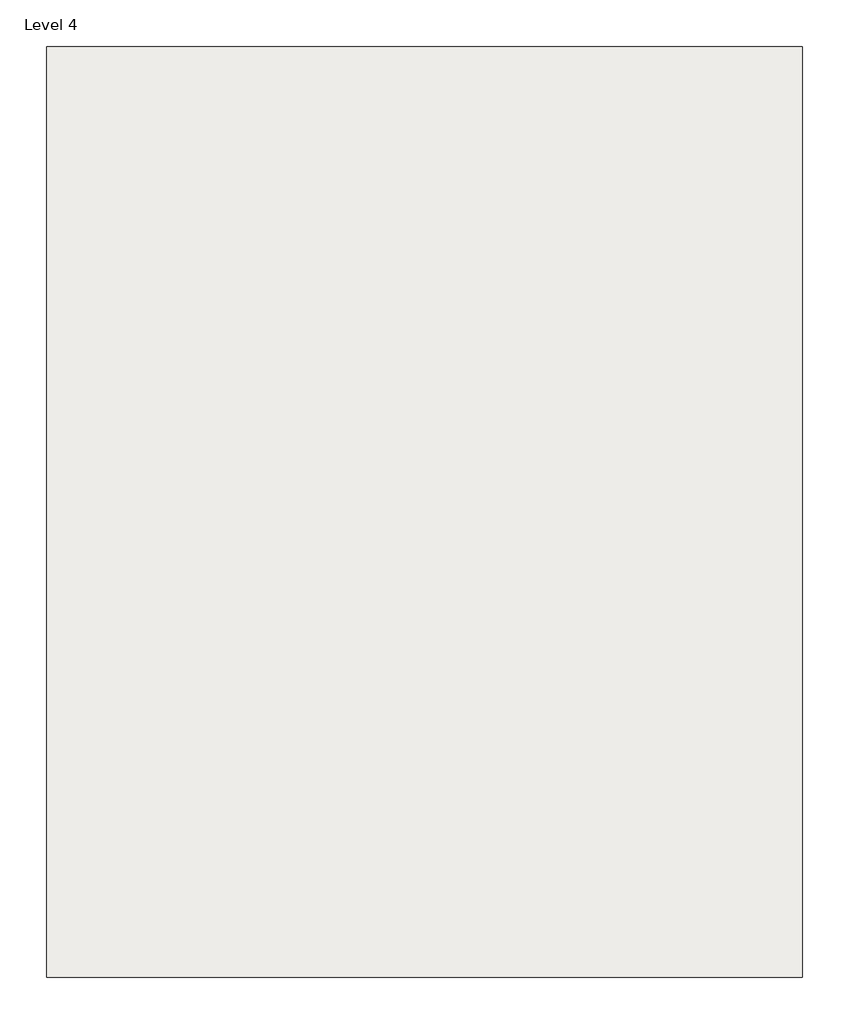
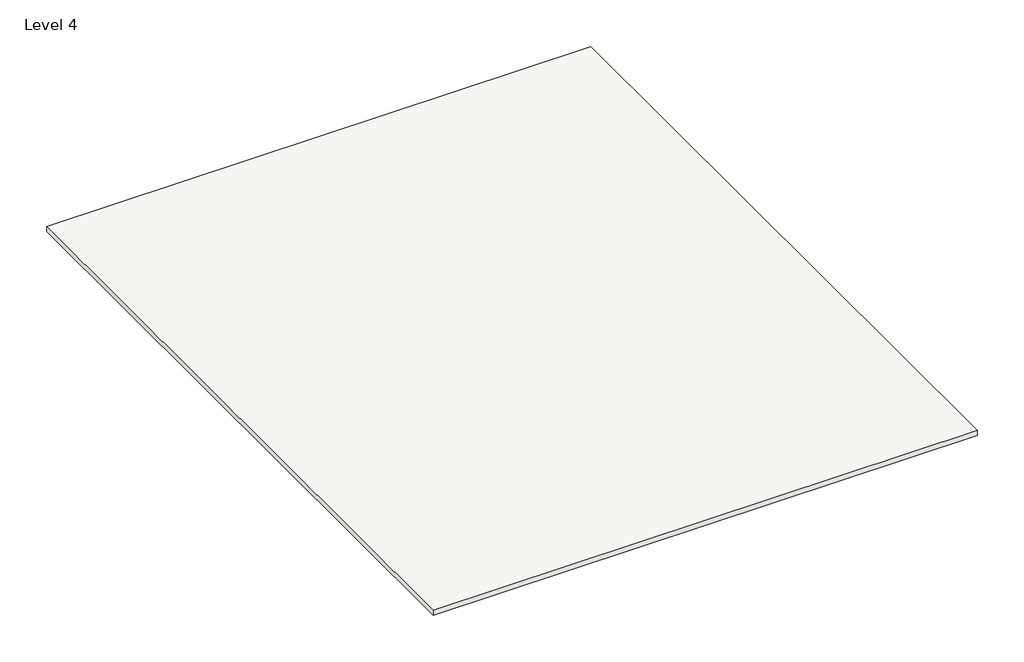
# One storey: 1 roof.
"""IFC4 building model written with IfcOpenShell, lengths in millimetres."""

from ifc_helpers import new_model, si_unit, frame, origin, place, context, project, spatial, polyline, outline, extrude, element, save

model = new_model("IFC4")

# Units and contexts
model_context = context("Model", 3, world=origin())
ifc_project = project(units=[si_unit("LENGTHUNIT", "METRE", prefix="MILLI")], contexts=[model_context])

# Site, building, storey
site = spatial("IfcSite", under=ifc_project)
building = spatial("IfcBuilding", under=site)
storey = spatial("IfcBuildingStorey", under=building, Name="Level 4", Elevation=6248.4)

# Roof
placement = place(None, origin())
element("IfcRoof", 1, ObjectType="6", at=placement, inside=storey, context=model_context, shape_type="SweptSolid", body=[
    extrude(outline(polyline([(74.1689082, 14608.7600271), (15923.7689082, 14608.7600271), (15923.7689082, -4898.4399729), (74.1689082, -4898.4399729), (74.1689082, 14608.7600271)])), frame((0.0, 0.0, 6248.4), z_axis=(0.0, 0.0, 1.0), x_axis=(1.0, 0.0, 0.0)), (0.0, 0.0, 1.0), 152.4),
])

save(model, "model.ifc")

# Revit data of these elements
# Type "6"
#   Assembly Code = "B1020"
#   Layers, outside or top first: 0' - 6" no material (function 1)
# Element 1 (IfcRoof, "6")
#   built-in parameter 1001705 = 21 (stored number, unit not read)
#   built-in parameter 1001710 = 33615
#   Phase Created = New Construction
#   Materials on its faces: "Default Roof"
# Materials
#   "Default Roof": colour RGB 88 101 114, transparency 0
